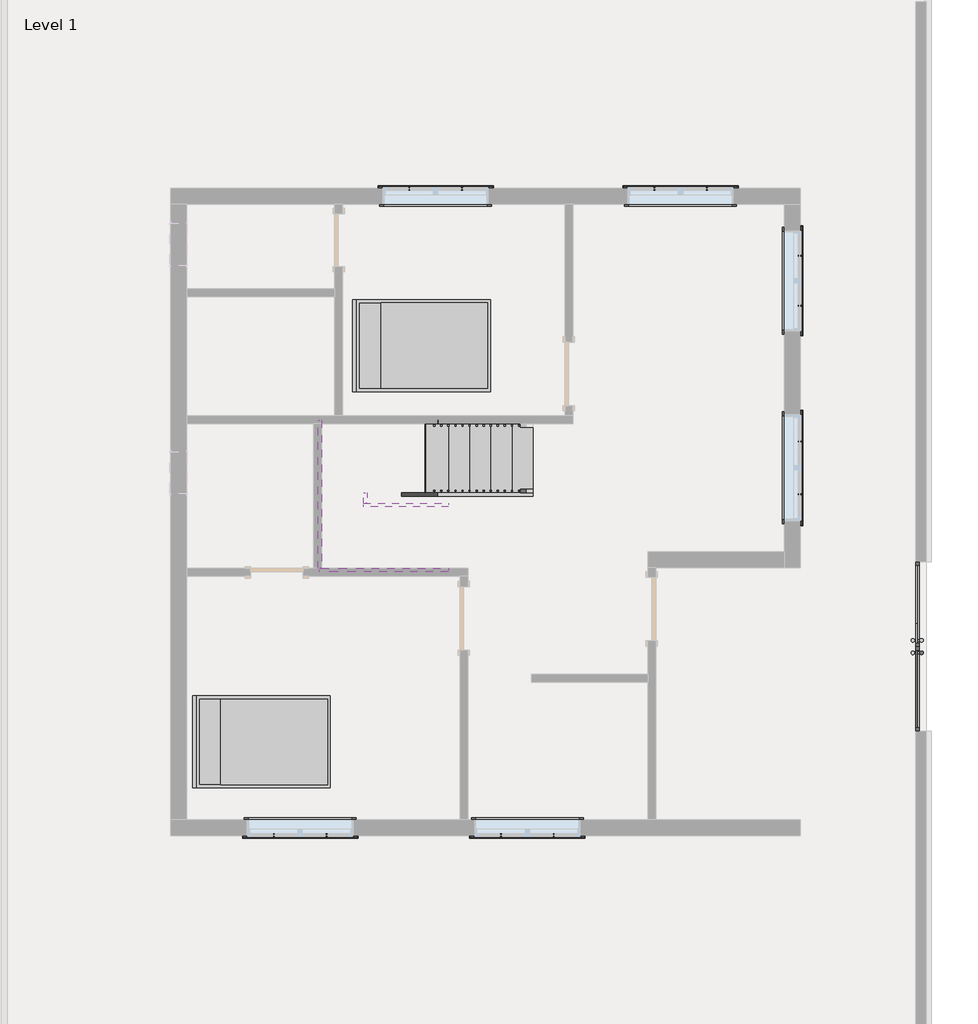
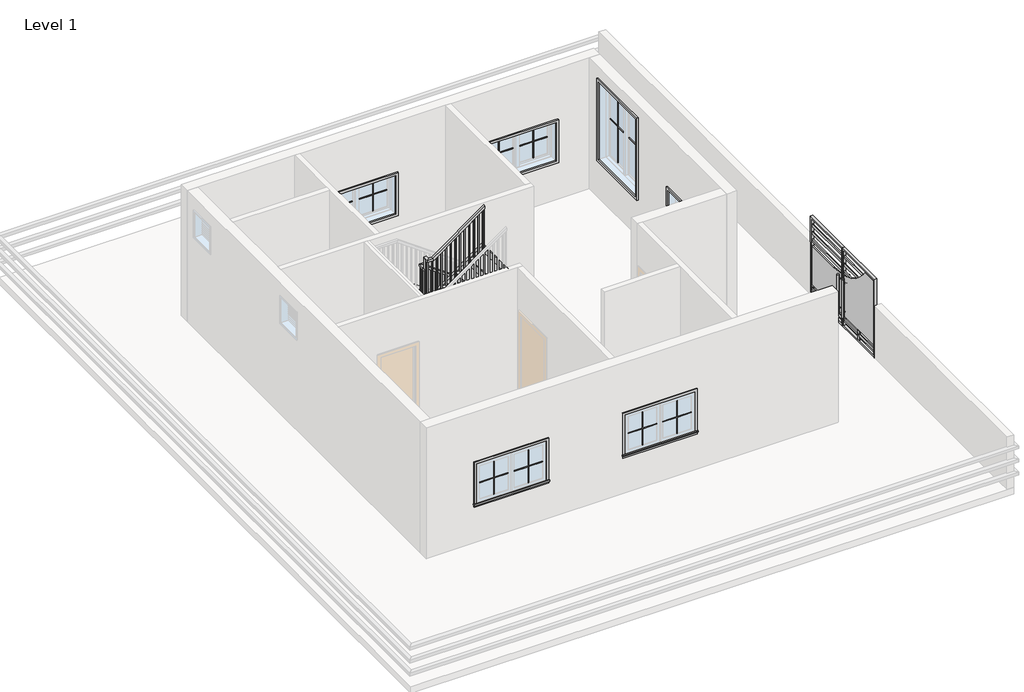
# One storey, part 3 of 3: 25 proxies, 6 members, 2 furniture elements, 1 railing, 1 stair flight.
"""IFC4 building model written with IfcOpenShell, lengths in millimetres."""

from ifc_helpers import new_model, si_unit, frame, origin, place, context, project, spatial, polyline, outline, extrude, faceted_brep, transform, mapped, element, save
from components import generic_models_113f6068, muntin_pattern_2x2_muntin_pattern_2x2_9352d081, muntin_pattern_2x2_muntin_pattern_2x2_5c2cbe28, muntin_pattern_2x2_muntin_pattern_2x2_bff912c5, muntin_pattern_2x2_muntin_pattern_2x2_c2194282, trim_window_exterior_flat_with_sill_979bde60, trim_window_exterior_flat_with_sill_e04b3088, trim_window_interior_flat_picture_frame_7883d11b, trim_window_interior_flat_picture_frame_2a7685fe, bed_17739_bed_17739_15c61121, stair_flight_46f16e2a

model = new_model("IFC4")

# Units and contexts
model_context = context("Model", 3, world=origin())
ifc_project = project(units=[si_unit("LENGTHUNIT", "METRE", prefix="MILLI")], contexts=[model_context])

# Site, building, storey
site = spatial("IfcSite", under=ifc_project)
building = spatial("IfcBuilding", under=site)
storey = spatial("IfcBuildingStorey", under=building, Name="Level 1", Elevation=0.0)

# Proxies
placement = place(None, origin())
generic_models_shape = generic_models_113f6068(model_context)
element("IfcBuildingElementProxy", 1, Name="Generic Models", at=placement, inside=storey, context=model_context, shape_type="MappedRepresentation", body=[
    mapped(generic_models_shape, transform((4942.185534, -2549.4042021, 0.0), x_axis=(0.0, 1.0, 0.0), y_axis=(-1.0, 0.0, 0.0), z_axis=(0.0, 0.0, 1.0))),
])
muntin_pattern_2x2_muntin_pattern_2x2_shape = muntin_pattern_2x2_muntin_pattern_2x2_9352d081(model_context)
element("IfcBuildingElementProxy", 2, Name="Muntin Pattern_2x2 : Muntin Pattern_2x2", ObjectType="Muntin Pattern_2x2 : Muntin Pattern_2x2", at=placement, inside=storey, context=model_context, shape_type="MappedRepresentation", body=[
    mapped(muntin_pattern_2x2_muntin_pattern_2x2_shape, transform((-3542.9505704, -5264.0292021, 984.25), x_axis=(-1.0, 0.0, 0.0), y_axis=(0.0, -1.0, 0.0), z_axis=(0.0, 0.0, 1.0))),
])
element("IfcBuildingElementProxy", 3, Name="Muntin Pattern_2x2 : Muntin Pattern_2x2", ObjectType="Muntin Pattern_2x2 : Muntin Pattern_2x2", at=placement, inside=storey, context=model_context, shape_type="MappedRepresentation", body=[
    mapped(muntin_pattern_2x2_muntin_pattern_2x2_shape, transform((-272.7005704, -5264.0292021, 984.25), x_axis=(-1.0, 0.0, 0.0), y_axis=(0.0, -1.0, 0.0), z_axis=(0.0, 0.0, 1.0))),
])
element("IfcBuildingElementProxy", 4, Name="Muntin Pattern_2x2 : Muntin Pattern_2x2", ObjectType="Muntin Pattern_2x2 : Muntin Pattern_2x2", at=placement, inside=storey, context=model_context, shape_type="MappedRepresentation", body=[
    mapped(muntin_pattern_2x2_muntin_pattern_2x2_shape, transform((3269.0119296, 401.7582979, 984.25), x_axis=(0.0, -1.0, 0.0), y_axis=(1.0, 0.0, 0.0), z_axis=(0.0, 0.0, 1.0))),
])
element("IfcBuildingElementProxy", 5, Name="Muntin Pattern_2x2 : Muntin Pattern_2x2", ObjectType="Muntin Pattern_2x2 : Muntin Pattern_2x2", at=placement, inside=storey, context=model_context, shape_type="MappedRepresentation", body=[
    mapped(muntin_pattern_2x2_muntin_pattern_2x2_shape, transform((1175.0994296, 4038.7207979, 984.25), x_axis=(1.0, 0.0, 0.0), y_axis=(0.0, 1.0, 0.0), z_axis=(0.0, 0.0, 1.0))),
])
element("IfcBuildingElementProxy", 6, Name="Muntin Pattern_2x2 : Muntin Pattern_2x2", ObjectType="Muntin Pattern_2x2 : Muntin Pattern_2x2", at=placement, inside=storey, context=model_context, shape_type="MappedRepresentation", body=[
    mapped(muntin_pattern_2x2_muntin_pattern_2x2_shape, transform((-2352.3255704, 4038.7207979, 984.25), x_axis=(1.0, 0.0, 0.0), y_axis=(0.0, 1.0, 0.0), z_axis=(0.0, 0.0, 1.0))),
])
muntin_pattern_2x2_muntin_pattern_2x2_2_shape = muntin_pattern_2x2_muntin_pattern_2x2_5c2cbe28(model_context)
element("IfcBuildingElementProxy", 7, Name="Muntin Pattern_2x2 : Muntin Pattern_2x2", ObjectType="Muntin Pattern_2x2 : Muntin Pattern_2x2", at=placement, inside=storey, context=model_context, shape_type="MappedRepresentation", body=[
    mapped(muntin_pattern_2x2_muntin_pattern_2x2_2_shape, transform((-4301.7755704, -5264.0292021, 984.25), x_axis=(1.0, 0.0, 0.0), y_axis=(0.0, 1.0, 0.0), z_axis=(0.0, 0.0, 1.0))),
])
element("IfcBuildingElementProxy", 8, Name="Muntin Pattern_2x2 : Muntin Pattern_2x2", ObjectType="Muntin Pattern_2x2 : Muntin Pattern_2x2", at=placement, inside=storey, context=model_context, shape_type="MappedRepresentation", body=[
    mapped(muntin_pattern_2x2_muntin_pattern_2x2_2_shape, transform((-1031.5255704, -5264.0292021, 984.25), x_axis=(1.0, 0.0, 0.0), y_axis=(0.0, 1.0, 0.0), z_axis=(0.0, 0.0, 1.0))),
])
element("IfcBuildingElementProxy", 9, Name="Muntin Pattern_2x2 : Muntin Pattern_2x2", ObjectType="Muntin Pattern_2x2 : Muntin Pattern_2x2", at=placement, inside=storey, context=model_context, shape_type="MappedRepresentation", body=[
    mapped(muntin_pattern_2x2_muntin_pattern_2x2_2_shape, transform((3269.0119296, -357.0667021, 984.25), x_axis=(0.0, 1.0, 0.0), y_axis=(-1.0, 0.0, 0.0), z_axis=(0.0, 0.0, 1.0))),
])
element("IfcBuildingElementProxy", 10, Name="Muntin Pattern_2x2 : Muntin Pattern_2x2", ObjectType="Muntin Pattern_2x2 : Muntin Pattern_2x2", at=placement, inside=storey, context=model_context, shape_type="MappedRepresentation", body=[
    mapped(muntin_pattern_2x2_muntin_pattern_2x2_2_shape, transform((1933.9244296, 4038.7207979, 984.25), x_axis=(-1.0, 0.0, 0.0), y_axis=(0.0, -1.0, 0.0), z_axis=(0.0, 0.0, 1.0))),
])
element("IfcBuildingElementProxy", 11, Name="Muntin Pattern_2x2 : Muntin Pattern_2x2", ObjectType="Muntin Pattern_2x2 : Muntin Pattern_2x2", at=placement, inside=storey, context=model_context, shape_type="MappedRepresentation", body=[
    mapped(muntin_pattern_2x2_muntin_pattern_2x2_2_shape, transform((-1593.5005704, 4038.7207979, 984.25), x_axis=(-1.0, 0.0, 0.0), y_axis=(0.0, -1.0, 0.0), z_axis=(0.0, 0.0, 1.0))),
])
muntin_pattern_2x2_muntin_pattern_2x2_3_shape = muntin_pattern_2x2_muntin_pattern_2x2_bff912c5(model_context)
element("IfcBuildingElementProxy", 12, Name="Muntin Pattern_2x2 : Muntin Pattern_2x2", ObjectType="Muntin Pattern_2x2 : Muntin Pattern_2x2", at=placement, inside=storey, context=model_context, shape_type="MappedRepresentation", body=[
    mapped(muntin_pattern_2x2_muntin_pattern_2x2_3_shape, transform((3269.0119296, 3075.1082979, 984.25), x_axis=(0.0, -1.0, 0.0), y_axis=(1.0, 0.0, 0.0), z_axis=(0.0, 0.0, 1.0))),
])
muntin_pattern_2x2_muntin_pattern_2x2_4_shape = muntin_pattern_2x2_muntin_pattern_2x2_c2194282(model_context)
element("IfcBuildingElementProxy", 13, Name="Muntin Pattern_2x2 : Muntin Pattern_2x2", ObjectType="Muntin Pattern_2x2 : Muntin Pattern_2x2", at=placement, inside=storey, context=model_context, shape_type="MappedRepresentation", body=[
    mapped(muntin_pattern_2x2_muntin_pattern_2x2_4_shape, transform((3269.0119296, 2354.3832979, 984.25), x_axis=(0.0, 1.0, 0.0), y_axis=(-1.0, 0.0, 0.0), z_axis=(0.0, 0.0, 1.0))),
])
trim_window_exterior_flat_with_sill_shape = trim_window_exterior_flat_with_sill_979bde60(model_context)
element("IfcBuildingElementProxy", 14, Name="Trim-Window-Exterior-Flat : with Sill", ObjectType="Trim-Window-Exterior-Flat : with Sill", at=placement, inside=storey, context=model_context, shape_type="MappedRepresentation", body=[
    mapped(trim_window_exterior_flat_with_sill_shape, transform((-3922.3630704, -5273.5542021, 1828.8), x_axis=(1.0, 0.0, 0.0), y_axis=(0.0, 0.0, 1.0), z_axis=(0.0, -1.0, 0.0))),
])
element("IfcBuildingElementProxy", 15, Name="Trim-Window-Exterior-Flat : with Sill", ObjectType="Trim-Window-Exterior-Flat : with Sill", at=placement, inside=storey, context=model_context, shape_type="MappedRepresentation", body=[
    mapped(trim_window_exterior_flat_with_sill_shape, transform((-652.1130704, -5273.5542021, 1828.8), x_axis=(1.0, 0.0, 0.0), y_axis=(0.0, 0.0, 1.0), z_axis=(0.0, -1.0, 0.0))),
])
element("IfcBuildingElementProxy", 16, Name="Trim-Window-Exterior-Flat : with Sill", ObjectType="Trim-Window-Exterior-Flat : with Sill", at=placement, inside=storey, context=model_context, shape_type="MappedRepresentation", body=[
    mapped(trim_window_exterior_flat_with_sill_shape, transform((3278.5369296, 22.3457979, 1828.8), x_axis=(0.0, 1.0, 0.0), y_axis=(0.0, 0.0, 1.0), z_axis=(1.0, 0.0, 0.0))),
])
element("IfcBuildingElementProxy", 17, Name="Trim-Window-Exterior-Flat : with Sill", ObjectType="Trim-Window-Exterior-Flat : with Sill", at=placement, inside=storey, context=model_context, shape_type="MappedRepresentation", body=[
    mapped(trim_window_exterior_flat_with_sill_shape, transform((1554.5119296, 4048.2457979, 1828.8), x_axis=(-1.0, 0.0, 0.0), y_axis=(0.0, 0.0, 1.0), z_axis=(0.0, 1.0, 0.0))),
])
element("IfcBuildingElementProxy", 18, Name="Trim-Window-Exterior-Flat : with Sill", ObjectType="Trim-Window-Exterior-Flat : with Sill", at=placement, inside=storey, context=model_context, shape_type="MappedRepresentation", body=[
    mapped(trim_window_exterior_flat_with_sill_shape, transform((-1972.9130704, 4048.2457979, 1828.8), x_axis=(-1.0, 0.0, 0.0), y_axis=(0.0, 0.0, 1.0), z_axis=(0.0, 1.0, 0.0))),
])
trim_window_exterior_flat_with_sill_2_shape = trim_window_exterior_flat_with_sill_e04b3088(model_context)
element("IfcBuildingElementProxy", 19, Name="Trim-Window-Exterior-Flat : with Sill", ObjectType="Trim-Window-Exterior-Flat : with Sill", at=placement, inside=storey, context=model_context, shape_type="MappedRepresentation", body=[
    mapped(trim_window_exterior_flat_with_sill_2_shape, transform((3278.5369296, 2714.7457979, 2743.2), x_axis=(0.0, 1.0, 0.0), y_axis=(0.0, 0.0, 1.0), z_axis=(1.0, 0.0, 0.0))),
])
trim_window_interior_flat_picture_frame_shape = trim_window_interior_flat_picture_frame_7883d11b(model_context)
element("IfcBuildingElementProxy", 20, Name="Trim-Window-Interior-Flat : Picture Frame", ObjectType="Trim-Window-Interior-Flat : Picture Frame", at=placement, inside=storey, context=model_context, shape_type="MappedRepresentation", body=[
    mapped(trim_window_interior_flat_picture_frame_shape, transform((-3922.3630704, -5044.9542021, 1828.8), x_axis=(-1.0, 0.0, 0.0), y_axis=(0.0, 0.0, 1.0), z_axis=(0.0, 1.0, 0.0))),
])
element("IfcBuildingElementProxy", 21, Name="Trim-Window-Interior-Flat : Picture Frame", ObjectType="Trim-Window-Interior-Flat : Picture Frame", at=placement, inside=storey, context=model_context, shape_type="MappedRepresentation", body=[
    mapped(trim_window_interior_flat_picture_frame_shape, transform((-652.1130704, -5044.9542021, 1828.8), x_axis=(-1.0, 0.0, 0.0), y_axis=(0.0, 0.0, 1.0), z_axis=(0.0, 1.0, 0.0))),
])
element("IfcBuildingElementProxy", 22, Name="Trim-Window-Interior-Flat : Picture Frame", ObjectType="Trim-Window-Interior-Flat : Picture Frame", at=placement, inside=storey, context=model_context, shape_type="MappedRepresentation", body=[
    mapped(trim_window_interior_flat_picture_frame_shape, transform((3049.9369296, 22.3457979, 1828.8), x_axis=(0.0, -1.0, 0.0), y_axis=(0.0, 0.0, 1.0), z_axis=(-1.0, 0.0, 0.0))),
])
element("IfcBuildingElementProxy", 23, Name="Trim-Window-Interior-Flat : Picture Frame", ObjectType="Trim-Window-Interior-Flat : Picture Frame", at=placement, inside=storey, context=model_context, shape_type="MappedRepresentation", body=[
    mapped(trim_window_interior_flat_picture_frame_shape, transform((1554.5119296, 3819.6457979, 1828.8), x_axis=(1.0, 0.0, 0.0), y_axis=(0.0, 0.0, 1.0), z_axis=(0.0, -1.0, 0.0))),
])
element("IfcBuildingElementProxy", 24, Name="Trim-Window-Interior-Flat : Picture Frame", ObjectType="Trim-Window-Interior-Flat : Picture Frame", at=placement, inside=storey, context=model_context, shape_type="MappedRepresentation", body=[
    mapped(trim_window_interior_flat_picture_frame_shape, transform((-1972.9130704, 3819.6457979, 1828.8), x_axis=(1.0, 0.0, 0.0), y_axis=(0.0, 0.0, 1.0), z_axis=(0.0, -1.0, 0.0))),
])
trim_window_interior_flat_picture_frame_2_shape = trim_window_interior_flat_picture_frame_2a7685fe(model_context)
element("IfcBuildingElementProxy", 25, Name="Trim-Window-Interior-Flat : Picture Frame", ObjectType="Trim-Window-Interior-Flat : Picture Frame", at=placement, inside=storey, context=model_context, shape_type="MappedRepresentation", body=[
    mapped(trim_window_interior_flat_picture_frame_2_shape, transform((3049.9369296, 2714.7457979, 2743.2), x_axis=(0.0, -1.0, 0.0), y_axis=(0.0, 0.0, 1.0), z_axis=(-1.0, 0.0, 0.0))),
])

# Furniture
bed_17739_bed_17739_shape = bed_17739_bed_17739_15c61121(model_context)
element("IfcFurniture", 26, ObjectType="Bed_17739 : Bed_17739", at=placement, inside=storey, context=model_context, shape_type="MappedRepresentation", body=[
    mapped(bed_17739_bed_17739_shape, transform((-4455.7630704, -3920.5467683, 0.0), x_axis=(0.0, 1.0, 0.0), y_axis=(-1.0, 0.0, 0.0), z_axis=(0.0, 0.0, 1.0))),
])
element("IfcFurniture", 27, ObjectType="Bed_17739 : Bed_17739", at=placement, inside=storey, context=model_context, shape_type="MappedRepresentation", body=[
    mapped(bed_17739_bed_17739_shape, transform((-2150.7130704, 1781.2957979, 0.0), x_axis=(0.0, 1.0, 0.0), y_axis=(-1.0, 0.0, 0.0), z_axis=(0.0, 0.0, 1.0))),
])

# Members
element("IfcMember", 28, ObjectType="Stringer - 2\" Width", at=placement, inside=storey, context=model_context, shape_type="SweptSolid", body=[
    extrude(outline(polyline([(0.0, -569.5630704), (223.0558696, -569.5630704), (1928.484441, -2957.1630704), (1553.9146208, -2957.1630704), (0.0, -781.6826013), (0.0, -569.5630704)])), frame((0.0, -384.0542021, 0.0), z_axis=(0.0, 1.0, 0.0), x_axis=(0.0, 0.0, 1.0)), (0.0, 0.0, 1.0), 50.8),
])
element("IfcMember", 29, ObjectType="Stringer - 2\" Width", at=placement, inside=storey, context=model_context, shape_type="SweptSolid", body=[
    extrude(outline(polyline([(-3007.9630704, -333.2542021), (-2957.1630704, -333.2542021), (-2957.1630704, -485.6542021), (-3007.9630704, -485.6542021), (-3007.9630704, -333.2542021)])), frame((0.0, 0.0, 1730.8285714), z_axis=(0.0, 0.0, 1.0), x_axis=(1.0, 0.0, 0.0)), (0.0, 0.0, 1.0), 304.8),
])
element("IfcMember", 30, ObjectType="Stringer - 2\" Width", at=placement, inside=storey, context=model_context, shape_type="SweptSolid", body=[
    extrude(outline(polyline([(2182.484441, -3007.9630704), (1807.9146208, -3007.9630704), (2678.7717636, -1788.7630704), (3053.3415838, -1788.7630704), (2182.484441, -3007.9630704)])), frame((0.0, -536.4542021, 0.0), z_axis=(0.0, 1.0, 0.0), x_axis=(0.0, 0.0, 1.0)), (0.0, 0.0, 1.0), 50.8),
])
element("IfcMember", 31, ObjectType="Stringer - 2\" Width", at=placement, inside=storey, context=model_context, shape_type="SweptSolid", body=[
    extrude(outline(polyline([(0.0, -569.5630704), (223.0558696, -569.5630704), (2035.6285714, -3107.1648531), (2035.6285714, -3617.5630704), (2025.6289065, -3617.5630704), (0.0, -781.6826013), (0.0, -569.5630704)])), frame((0.0, 657.3457979, 0.0), z_axis=(0.0, 1.0, 0.0), x_axis=(0.0, 0.0, 1.0)), (0.0, 0.0, 1.0), 50.8),
])
element("IfcMember", 32, ObjectType="Stringer - 2\" Width", at=placement, inside=storey, context=model_context, shape_type="SweptSolid", body=[
    extrude(outline(polyline([(-3668.3630704, 708.1457979), (-3617.5630704, 708.1457979), (-3617.5630704, -1425.4542021), (-3668.3630704, -1425.4542021), (-3668.3630704, 708.1457979)])), frame((0.0, 0.0, 1730.8285714), z_axis=(0.0, 0.0, 1.0), x_axis=(1.0, 0.0, 0.0)), (0.0, 0.0, 1.0), 304.8),
])
element("IfcMember", 33, ObjectType="Stringer - 2\" Width", at=placement, inside=storey, context=model_context, shape_type="SweptSolid", body=[
    extrude(outline(polyline([(1730.8285714, -3115.8835396), (2678.7717636, -1788.7630704), (3053.3415838, -1788.7630704), (1730.8285714, -3640.2812878), (1730.8285714, -3115.8835396)])), frame((0.0, -1476.2542021, 0.0), z_axis=(0.0, 1.0, 0.0), x_axis=(0.0, 0.0, 1.0)), (0.0, 0.0, 1.0), 50.8),
])

# Railing
element("IfcRailing", 34, ObjectType="Handrail - Rectangular", at=placement, inside=storey, context=model_context, shape_type="SolidModel", body=[
    faceted_brep([(-569.5630704, -333.2542021, 1132.1142857), (-569.5630704, -333.2542021, 1069.6859823), (-569.5630704, -282.4542021, 1069.6859823), (-569.5630704, -282.4542021, 1132.1142857), (-2931.7630704, -333.2542021, 2819.4), (-2982.5630704, -333.2542021, 2793.2574109), (-2982.5630704, -282.4542021, 2793.2574109), (-2931.7630704, -282.4542021, 2819.4), (-2931.7630704, -333.2542021, 2873.8285714), (-2982.5630704, -333.2542021, 2823.0285714), (-2982.5630704, -282.4542021, 2823.0285714), (-2931.7630704, -282.4542021, 2873.8285714), (-3007.9630704, -333.2542021, 2873.8285714), (-3007.9630704, -333.2542021, 2823.0285714), (-3058.7630704, -282.4542021, 2823.0285714), (-3058.7630704, -282.4542021, 2873.8285714), (-3007.9630704, -409.4542021, 2873.8285714), (-3007.9630704, -409.4542021, 2823.0285714), (-3058.7630704, -409.4542021, 2823.0285714), (-3058.7630704, -409.4542021, 2873.8285714), (-3007.9630704, -460.2542021, 2873.8285714), (-3007.9630704, -511.0542021, 2823.0285714), (-3058.7630704, -511.0542021, 2823.0285714), (-3058.7630704, -460.2542021, 2873.8285714), (-3007.9630704, -460.2542021, 3145.9714286), (-3007.9630704, -511.0542021, 3095.1714286), (-3058.7630704, -511.0542021, 3095.1714286), (-3058.7630704, -460.2542021, 3145.9714286), (-3007.9630704, -536.4542021, 3145.9714286), (-3007.9630704, -536.4542021, 3095.1714286), (-3058.7630704, -587.2542021, 3095.1714286), (-3058.7630704, -587.2542021, 3145.9714286), (-2931.7630704, -536.4542021, 3145.9714286), (-2915.4834457, -536.4542021, 3095.1714286), (-2915.4834457, -587.2542021, 3095.1714286), (-2931.7630704, -587.2542021, 3145.9714286), (-1788.7630704, -536.4542021, 3962.4), (-1788.7630704, -587.2542021, 3962.4), (-1788.7630704, -587.2542021, 3899.9716966), (-1788.7630704, -536.4542021, 3899.9716966)], [[[0, 1, 2, 3]], [[1, 0, 4, 5]], [[2, 1, 5, 6]], [[3, 2, 6, 7]], [[0, 3, 7, 4]], [[5, 4, 8, 9]], [[6, 5, 9, 10]], [[7, 6, 10, 11]], [[4, 7, 11, 8]], [[9, 8, 12, 13]], [[10, 9, 13, 14]], [[11, 10, 14, 15]], [[8, 11, 15, 12]], [[13, 12, 16, 17]], [[14, 13, 17, 18]], [[15, 14, 18, 19]], [[12, 15, 19, 16]], [[17, 16, 20, 21]], [[18, 17, 21, 22]], [[19, 18, 22, 23]], [[16, 19, 23, 20]], [[21, 20, 24, 25]], [[22, 21, 25, 26]], [[23, 22, 26, 27]], [[20, 23, 27, 24]], [[25, 24, 28, 29]], [[26, 25, 29, 30]], [[27, 26, 30, 31]], [[24, 27, 31, 28]], [[29, 28, 32, 33]], [[30, 29, 33, 34]], [[31, 30, 34, 35]], [[28, 31, 35, 32]], [[36, 37, 38, 39]], [[33, 32, 36, 39]], [[34, 33, 39, 38]], [[35, 34, 38, 37]], [[32, 35, 37, 36]]]),
    extrude(outline(polyline([(3875.0252681, -1823.6880704), (2830.2857143, -1823.6880704), (2830.2857143, -1804.6380704), (3888.6324109, -1804.6380704), (3875.0252681, -1823.6880704)])), frame((0.0, -571.3792021, 0.0), z_axis=(0.0, 1.0, 0.0), x_axis=(0.0, 0.0, 1.0)), (0.0, 0.0, 1.0), 19.05),
    extrude(outline(polyline([(3802.4538395, -1925.2880704), (2830.2857143, -1925.2880704), (2830.2857143, -1906.2380704), (3816.0609823, -1906.2380704), (3802.4538395, -1925.2880704)])), frame((0.0, -571.3792021, 0.0), z_axis=(0.0, 1.0, 0.0), x_axis=(0.0, 0.0, 1.0)), (0.0, 0.0, 1.0), 19.05),
    extrude(outline(polyline([(3729.8824109, -2026.8880704), (2830.2857143, -2026.8880704), (2830.2857143, -2007.8380704), (3743.4895538, -2007.8380704), (3729.8824109, -2026.8880704)])), frame((0.0, -571.3792021, 0.0), z_axis=(0.0, 1.0, 0.0), x_axis=(0.0, 0.0, 1.0)), (0.0, 0.0, 1.0), 19.05),
    extrude(outline(polyline([(3657.3109823, -2128.4880704), (2612.5714286, -2128.4880704), (2612.5714286, -2109.4380704), (3670.9181252, -2109.4380704), (3657.3109823, -2128.4880704)])), frame((0.0, -571.3792021, 0.0), z_axis=(0.0, 1.0, 0.0), x_axis=(0.0, 0.0, 1.0)), (0.0, 0.0, 1.0), 19.05),
    extrude(outline(polyline([(3584.7395538, -2230.0880704), (2612.5714286, -2230.0880704), (2612.5714286, -2211.0380704), (3598.3466966, -2211.0380704), (3584.7395538, -2230.0880704)])), frame((0.0, -571.3792021, 0.0), z_axis=(0.0, 1.0, 0.0), x_axis=(0.0, 0.0, 1.0)), (0.0, 0.0, 1.0), 19.05),
    extrude(outline(polyline([(3512.1681252, -2331.6880704), (2612.5714286, -2331.6880704), (2612.5714286, -2312.6380704), (3525.7752681, -2312.6380704), (3512.1681252, -2331.6880704)])), frame((0.0, -571.3792021, 0.0), z_axis=(0.0, 1.0, 0.0), x_axis=(0.0, 0.0, 1.0)), (0.0, 0.0, 1.0), 19.05),
    extrude(outline(polyline([(3439.5966966, -2433.2880704), (2394.8571429, -2433.2880704), (2394.8571429, -2414.2380704), (3453.2038395, -2414.2380704), (3439.5966966, -2433.2880704)])), frame((0.0, -571.3792021, 0.0), z_axis=(0.0, 1.0, 0.0), x_axis=(0.0, 0.0, 1.0)), (0.0, 0.0, 1.0), 19.05),
    extrude(outline(polyline([(3367.0252681, -2534.8880704), (2394.8571429, -2534.8880704), (2394.8571429, -2515.8380704), (3380.6324109, -2515.8380704), (3367.0252681, -2534.8880704)])), frame((0.0, -571.3792021, 0.0), z_axis=(0.0, 1.0, 0.0), x_axis=(0.0, 0.0, 1.0)), (0.0, 0.0, 1.0), 19.05),
    extrude(outline(polyline([(3294.4538395, -2636.4880704), (2394.8571429, -2636.4880704), (2394.8571429, -2617.4380704), (3308.0609823, -2617.4380704), (3294.4538395, -2636.4880704)])), frame((0.0, -571.3792021, 0.0), z_axis=(0.0, 1.0, 0.0), x_axis=(0.0, 0.0, 1.0)), (0.0, 0.0, 1.0), 19.05),
    extrude(outline(polyline([(3221.8824109, -2738.0880704), (2177.1428571, -2738.0880704), (2177.1428571, -2719.0380704), (3235.4895538, -2719.0380704), (3221.8824109, -2738.0880704)])), frame((0.0, -571.3792021, 0.0), z_axis=(0.0, 1.0, 0.0), x_axis=(0.0, 0.0, 1.0)), (0.0, 0.0, 1.0), 19.05),
    extrude(outline(polyline([(3149.3109823, -2839.6880704), (2177.1428571, -2839.6880704), (2177.1428571, -2820.6380704), (3162.9181252, -2820.6380704), (3149.3109823, -2839.6880704)])), frame((0.0, -571.3792021, 0.0), z_axis=(0.0, 1.0, 0.0), x_axis=(0.0, 0.0, 1.0)), (0.0, 0.0, 1.0), 19.05),
    extrude(outline(polyline([(3076.7395538, -2941.2880704), (2177.1428571, -2941.2880704), (2177.1428571, -2922.2380704), (3090.3466966, -2922.2380704), (3076.7395538, -2941.2880704)])), frame((0.0, -571.3792021, 0.0), z_axis=(0.0, 1.0, 0.0), x_axis=(0.0, 0.0, 1.0)), (0.0, 0.0, 1.0), 19.05),
    extrude(outline(polyline([(-3023.8380704, -501.5292021), (-3023.8380704, -520.5792021), (-3042.8880704, -520.5792021), (-3042.8880704, -501.5292021), (-3023.8380704, -501.5292021)])), frame((0.0, 0.0, 1959.4285714), z_axis=(0.0, 0.0, 1.0), x_axis=(1.0, 0.0, 0.0)), (0.0, 0.0, 1.0), 1135.7428571),
    extrude(outline(polyline([(-3023.8380704, -399.9292021), (-3023.8380704, -418.9792021), (-3042.8880704, -418.9792021), (-3042.8880704, -399.9292021), (-3023.8380704, -399.9292021)])), frame((0.0, 0.0, 1959.4285714), z_axis=(0.0, 0.0, 1.0), x_axis=(1.0, 0.0, 0.0)), (0.0, 0.0, 1.0), 863.6),
    extrude(outline(polyline([(-2998.4380704, -317.3792021), (-3017.4880704, -317.3792021), (-3017.4880704, -298.3292021), (-2998.4380704, -298.3292021), (-2998.4380704, -317.3792021)])), frame((0.0, 0.0, 1959.4285714), z_axis=(0.0, 0.0, 1.0), x_axis=(1.0, 0.0, 0.0)), (0.0, 0.0, 1.0), 863.6),
    extrude(outline(polyline([(2745.6324109, -2915.8880704), (1741.7142857, -2915.8880704), (1741.7142857, -2896.8380704), (2732.0252681, -2896.8380704), (2745.6324109, -2915.8880704)])), frame((0.0, -317.3792021, 0.0), z_axis=(0.0, 1.0, 0.0), x_axis=(0.0, 0.0, 1.0)), (0.0, 0.0, 1.0), 19.05),
    extrude(outline(polyline([(2673.0609823, -2814.2880704), (1741.7142857, -2814.2880704), (1741.7142857, -2795.2380704), (2659.4538395, -2795.2380704), (2673.0609823, -2814.2880704)])), frame((0.0, -317.3792021, 0.0), z_axis=(0.0, 1.0, 0.0), x_axis=(0.0, 0.0, 1.0)), (0.0, 0.0, 1.0), 19.05),
    extrude(outline(polyline([(2600.4895538, -2712.6880704), (1741.7142857, -2712.6880704), (1741.7142857, -2693.6380704), (2586.8824109, -2693.6380704), (2600.4895538, -2712.6880704)])), frame((0.0, -317.3792021, 0.0), z_axis=(0.0, 1.0, 0.0), x_axis=(0.0, 0.0, 1.0)), (0.0, 0.0, 1.0), 19.05),
    extrude(outline(polyline([(2527.9181252, -2611.0880704), (1524.0, -2611.0880704), (1524.0, -2592.0380704), (2514.3109823, -2592.0380704), (2527.9181252, -2611.0880704)])), frame((0.0, -317.3792021, 0.0), z_axis=(0.0, 1.0, 0.0), x_axis=(0.0, 0.0, 1.0)), (0.0, 0.0, 1.0), 19.05),
    extrude(outline(polyline([(2455.3466966, -2509.4880704), (1524.0, -2509.4880704), (1524.0, -2490.4380704), (2441.7395538, -2490.4380704), (2455.3466966, -2509.4880704)])), frame((0.0, -317.3792021, 0.0), z_axis=(0.0, 1.0, 0.0), x_axis=(0.0, 0.0, 1.0)), (0.0, 0.0, 1.0), 19.05),
    extrude(outline(polyline([(2382.7752681, -2407.8880704), (1524.0, -2407.8880704), (1524.0, -2388.8380704), (2369.1681252, -2388.8380704), (2382.7752681, -2407.8880704)])), frame((0.0, -317.3792021, 0.0), z_axis=(0.0, 1.0, 0.0), x_axis=(0.0, 0.0, 1.0)), (0.0, 0.0, 1.0), 19.05),
    extrude(outline(polyline([(2310.2038395, -2306.2880704), (1306.2857143, -2306.2880704), (1306.2857143, -2287.2380704), (2296.5966966, -2287.2380704), (2310.2038395, -2306.2880704)])), frame((0.0, -317.3792021, 0.0), z_axis=(0.0, 1.0, 0.0), x_axis=(0.0, 0.0, 1.0)), (0.0, 0.0, 1.0), 19.05),
    extrude(outline(polyline([(2237.6324109, -2204.6880704), (1306.2857143, -2204.6880704), (1306.2857143, -2185.6380704), (2224.0252681, -2185.6380704), (2237.6324109, -2204.6880704)])), frame((0.0, -317.3792021, 0.0), z_axis=(0.0, 1.0, 0.0), x_axis=(0.0, 0.0, 1.0)), (0.0, 0.0, 1.0), 19.05),
    extrude(outline(polyline([(2165.0609823, -2103.0880704), (1306.2857143, -2103.0880704), (1306.2857143, -2084.0380704), (2151.4538395, -2084.0380704), (2165.0609823, -2103.0880704)])), frame((0.0, -317.3792021, 0.0), z_axis=(0.0, 1.0, 0.0), x_axis=(0.0, 0.0, 1.0)), (0.0, 0.0, 1.0), 19.05),
    extrude(outline(polyline([(2092.4895538, -2001.4880704), (1088.5714286, -2001.4880704), (1088.5714286, -1982.4380704), (2078.8824109, -1982.4380704), (2092.4895538, -2001.4880704)])), frame((0.0, -317.3792021, 0.0), z_axis=(0.0, 1.0, 0.0), x_axis=(0.0, 0.0, 1.0)), (0.0, 0.0, 1.0), 19.05),
    extrude(outline(polyline([(2019.9181252, -1899.8880704), (1088.5714286, -1899.8880704), (1088.5714286, -1880.8380704), (2006.3109823, -1880.8380704), (2019.9181252, -1899.8880704)])), frame((0.0, -317.3792021, 0.0), z_axis=(0.0, 1.0, 0.0), x_axis=(0.0, 0.0, 1.0)), (0.0, 0.0, 1.0), 19.05),
    extrude(outline(polyline([(1947.3466966, -1798.2880704), (1088.5714286, -1798.2880704), (1088.5714286, -1779.2380704), (1933.7395538, -1779.2380704), (1947.3466966, -1798.2880704)])), frame((0.0, -317.3792021, 0.0), z_axis=(0.0, 1.0, 0.0), x_axis=(0.0, 0.0, 1.0)), (0.0, 0.0, 1.0), 19.05),
    extrude(outline(polyline([(1874.7752681, -1696.6880704), (870.8571429, -1696.6880704), (870.8571429, -1677.6380704), (1861.1681252, -1677.6380704), (1874.7752681, -1696.6880704)])), frame((0.0, -317.3792021, 0.0), z_axis=(0.0, 1.0, 0.0), x_axis=(0.0, 0.0, 1.0)), (0.0, 0.0, 1.0), 19.05),
    extrude(outline(polyline([(1802.2038395, -1595.0880704), (870.8571429, -1595.0880704), (870.8571429, -1576.0380704), (1788.5966966, -1576.0380704), (1802.2038395, -1595.0880704)])), frame((0.0, -317.3792021, 0.0), z_axis=(0.0, 1.0, 0.0), x_axis=(0.0, 0.0, 1.0)), (0.0, 0.0, 1.0), 19.05),
    extrude(outline(polyline([(1729.6324109, -1493.4880704), (870.8571429, -1493.4880704), (870.8571429, -1474.4380704), (1716.0252681, -1474.4380704), (1729.6324109, -1493.4880704)])), frame((0.0, -317.3792021, 0.0), z_axis=(0.0, 1.0, 0.0), x_axis=(0.0, 0.0, 1.0)), (0.0, 0.0, 1.0), 19.05),
    extrude(outline(polyline([(1657.0609823, -1391.8880704), (653.1428571, -1391.8880704), (653.1428571, -1372.8380704), (1643.4538395, -1372.8380704), (1657.0609823, -1391.8880704)])), frame((0.0, -317.3792021, 0.0), z_axis=(0.0, 1.0, 0.0), x_axis=(0.0, 0.0, 1.0)), (0.0, 0.0, 1.0), 19.05),
    extrude(outline(polyline([(1584.4895538, -1290.2880704), (653.1428571, -1290.2880704), (653.1428571, -1271.2380704), (1570.8824109, -1271.2380704), (1584.4895538, -1290.2880704)])), frame((0.0, -317.3792021, 0.0), z_axis=(0.0, 1.0, 0.0), x_axis=(0.0, 0.0, 1.0)), (0.0, 0.0, 1.0), 19.05),
    extrude(outline(polyline([(1511.9181252, -1188.6880704), (653.1428571, -1188.6880704), (653.1428571, -1169.6380704), (1498.3109823, -1169.6380704), (1511.9181252, -1188.6880704)])), frame((0.0, -317.3792021, 0.0), z_axis=(0.0, 1.0, 0.0), x_axis=(0.0, 0.0, 1.0)), (0.0, 0.0, 1.0), 19.05),
    extrude(outline(polyline([(1439.3466966, -1087.0880704), (435.4285714, -1087.0880704), (435.4285714, -1068.0380704), (1425.7395538, -1068.0380704), (1439.3466966, -1087.0880704)])), frame((0.0, -317.3792021, 0.0), z_axis=(0.0, 1.0, 0.0), x_axis=(0.0, 0.0, 1.0)), (0.0, 0.0, 1.0), 19.05),
    extrude(outline(polyline([(1366.7752681, -985.4880704), (435.4285714, -985.4880704), (435.4285714, -966.4380704), (1353.1681252, -966.4380704), (1366.7752681, -985.4880704)])), frame((0.0, -317.3792021, 0.0), z_axis=(0.0, 1.0, 0.0), x_axis=(0.0, 0.0, 1.0)), (0.0, 0.0, 1.0), 19.05),
    extrude(outline(polyline([(1294.2038395, -883.8880704), (435.4285714, -883.8880704), (435.4285714, -864.8380704), (1280.5966966, -864.8380704), (1294.2038395, -883.8880704)])), frame((0.0, -317.3792021, 0.0), z_axis=(0.0, 1.0, 0.0), x_axis=(0.0, 0.0, 1.0)), (0.0, 0.0, 1.0), 19.05),
    extrude(outline(polyline([(1221.6324109, -782.2880704), (217.7142857, -782.2880704), (217.7142857, -763.2380704), (1208.0252681, -763.2380704), (1221.6324109, -782.2880704)])), frame((0.0, -317.3792021, 0.0), z_axis=(0.0, 1.0, 0.0), x_axis=(0.0, 0.0, 1.0)), (0.0, 0.0, 1.0), 19.05),
    extrude(outline(polyline([(1149.0609823, -680.6880704), (217.7142857, -680.6880704), (217.7142857, -661.6380704), (1135.4538395, -661.6380704), (1149.0609823, -680.6880704)])), frame((0.0, -317.3792021, 0.0), z_axis=(0.0, 1.0, 0.0), x_axis=(0.0, 0.0, 1.0)), (0.0, 0.0, 1.0), 19.05),
    extrude(outline(polyline([(-3023.8380704, -552.3292021), (-3023.8380704, -571.3792021), (-3042.8880704, -571.3792021), (-3042.8880704, -552.3292021), (-3023.8380704, -552.3292021)])), frame((0.0, 0.0, 1959.4285714), z_axis=(0.0, 0.0, 1.0), x_axis=(1.0, 0.0, 0.0)), (0.0, 0.0, 1.0), 1135.7428571),
    extrude(outline(polyline([(-3023.8380704, -317.3792021), (-3042.8880704, -317.3792021), (-3042.8880704, -298.3292021), (-3023.8380704, -298.3292021), (-3023.8380704, -317.3792021)])), frame((0.0, 0.0, 1959.4285714), z_axis=(0.0, 0.0, 1.0), x_axis=(1.0, 0.0, 0.0)), (0.0, 0.0, 1.0), 863.6),
    extrude(outline(polyline([(3886.3645538, -1807.8130704), (2830.2857143, -1807.8130704), (2830.2857143, -1788.7630704), (3899.9716966, -1788.7630704), (3886.3645538, -1807.8130704)])), frame((0.0, -571.3792021, 0.0), z_axis=(0.0, 1.0, 0.0), x_axis=(0.0, 0.0, 1.0)), (0.0, 0.0, 1.0), 19.05),
    extrude(outline(polyline([(1083.2931252, -588.6130704), (217.7142857, -588.6130704), (217.7142857, -569.5630704), (1069.6859823, -569.5630704), (1083.2931252, -588.6130704)])), frame((0.0, -317.3792021, 0.0), z_axis=(0.0, 1.0, 0.0), x_axis=(0.0, 0.0, 1.0)), (0.0, 0.0, 1.0), 19.05),
])

# Stair flight
stair_flight_shape = stair_flight_46f16e2a(model_context)
element("IfcStairFlight", 35, ObjectType="2\" Tread 1\" Nosing 1/4\" Riser", at=placement, inside=storey, context=model_context, shape_type="MappedRepresentation", body=[
    mapped(stair_flight_shape, transform((0.0, 0.0, 0.0), x_axis=(1.0, 0.0, 0.0), y_axis=(0.0, 1.0, 0.0), z_axis=(0.0, 0.0, 1.0))),
])

save(model, "model.ifc")

# Revit data of these elements
# Type
#   sheet = none
#   pipe = none
#   handal = none
#   faram = none
#   Default Elevation = 0
# Type "Muntin Pattern_2x2 : Muntin Pattern_2x2"
#   Width [instance default] = 4' - 0"
#   Thickness = 0' - 0 1/2"
#   Height [instance default] = 4' - 0"
#   Distance = 0' - 0 3/4"
#   Interior Material [instance default] = none
#   Exterior Material [instance default] = none
#   Default Elevation = 0
# Type "Trim-Window-Exterior-Flat : with Sill"
#   Trim Width = 0' - 2 1/4"
#   Trim Thickness_Picture Frame = 0' - 1 1/4"
#   Trim Thickness_with Sill = 0' - 0 3/4"
#   Sill Thickness = 0' - 1 1/4"
#   Opening Width [instance default] = 2' - 0"
#   Opening Height [instance default] = 3' - 0"
#   Default Elevation = 4' - 0"
#   Sill = yes
#   Picture Frame = no
#   Trim Material [instance default] = none
# Type "Trim-Window-Interior-Flat : Picture Frame"
#   Trim Thickness_Picture Frame = 0' - 1 1/4"
#   Trim Width = 0' - 2 1/4"
#   Trim Thickness_with Sill = 0' - 0 3/4"
#   Sill Thickness = 0' - 1 1/4"
#   Opening Width [instance default] = 2' - 0"
#   Opening Height [instance default] = 3' - 0"
#   Default Elevation = 4' - 0"
#   Sill = no
#   Picture Frame = yes
#   Trim Material [instance default] = none
# Type "Bed_17739 : Bed_17739"
#   Default Elevation = 0
# Type "Handrail - Rectangular"
#   Assembly Code = "C2010400"
#   built-in parameter 1008612 = 0.0416667 (stored number, unit not read)
#   built-in parameter 1008611 = 0.0416667 (stored number, unit not read)
#   built-in parameter 1008609 = 0.333333 (stored number, unit not read)
#   built-in parameter 1008604 = 0.166667 (stored number, unit not read)
#   built-in parameter 1008603 = 0.166667 (stored number, unit not read)
#   Railing Height = 3' - 0"
#   built-in parameter 1008630 = 2
#   built-in parameter 1008610 = 2
#   built-in parameter 1008618 = Baluster - Square : 3/4"
# Element 1 (IfcBuildingElementProxy)
#   Phase Created = New Construction
# Elements 2, 3, 4, 5, 6, 7, 8, 9, 10, 11 (IfcBuildingElementProxy, "Muntin Pattern_2x2 : Muntin Pattern_2x2")
#   Width = 2' - 0 5/8"
#   Height = 2' - 6 1/2"
#   Interior Material = Wood - Stained
#   Exterior Material = Clad - White
#   Phase Created = New Construction
#   Materials on its faces: "Clad - White", "Wood - Stained"
# Elements 12, 13 (IfcBuildingElementProxy, "Muntin Pattern_2x2 : Muntin Pattern_2x2")
#   Width = 1' - 11 1/8"
#   Height = 5' - 6 1/2"
#   Interior Material = Wood - Stained
#   Exterior Material = Clad - White
#   Phase Created = New Construction
#   Materials on its faces: "Clad - White", "Wood - Stained"
# Elements 14, 15, 16, 17, 18 (IfcBuildingElementProxy, "Trim-Window-Exterior-Flat : with Sill")
#   Opening Width = 5' - 0"
#   Opening Height = 3' - 0"
#   Trim Material = Clad - White
#   Phase Created = New Construction
#   Materials on its faces: "Clad - White"
# Element 19 (IfcBuildingElementProxy, "Trim-Window-Exterior-Flat : with Sill")
#   Opening Width = 4' - 9"
#   Opening Height = 6' - 0"
#   Trim Material = Clad - White
#   Phase Created = New Construction
#   Materials on its faces: "Clad - White"
# Elements 20, 21, 22, 23, 24 (IfcBuildingElementProxy, "Trim-Window-Interior-Flat : Picture Frame")
#   Opening Width = 5' - 0"
#   Opening Height = 3' - 0"
#   Trim Material = Wood - Stained
#   Phase Created = New Construction
#   Materials on its faces: "Wood - Stained"
# Element 25 (IfcBuildingElementProxy, "Trim-Window-Interior-Flat : Picture Frame")
#   Opening Width = 4' - 9"
#   Opening Height = 6' - 0"
#   Trim Material = Wood - Stained
#   Phase Created = New Construction
#   Materials on its faces: "Wood - Stained"
# Elements 26, 27 (IfcFurniture, "Bed_17739 : Bed_17739")
#   Phase Created = New Construction
#   Materials on its faces: "legs", "sheets", "bed frame", "Blanket"
# Elements 28, 29, 30, 31, 32, 33 (IfcMember, "Stringer - 2\" Width")
#   Phase Created = New Construction
# Element 34 (IfcRailing, "Handrail - Rectangular")
#   Phase Created = New Construction
# Element 35 (IfcStairFlight, "2\" Tread 1\" Nosing 1/4\" Riser")
#   Phase Created = New Construction
# Materials
#   "Clad - White": class "Wood", colour RGB 242 242 238, transparency 0, Cost = 0
#   "Wood - Stained": class "Wood", colour RGB 224 178 126, transparency 0, Cost = 0
#   "legs": colour RGB 90 73 37, transparency 0, Cost = 0
#   "sheets": colour RGB 200 195 176, transparency 0, Cost = 0
#   "bed frame": colour RGB 90 73 37, transparency 0, Cost = 0
#   "Blanket": class "System", colour RGB 59 0 1, transparency 0, Cost = 0
